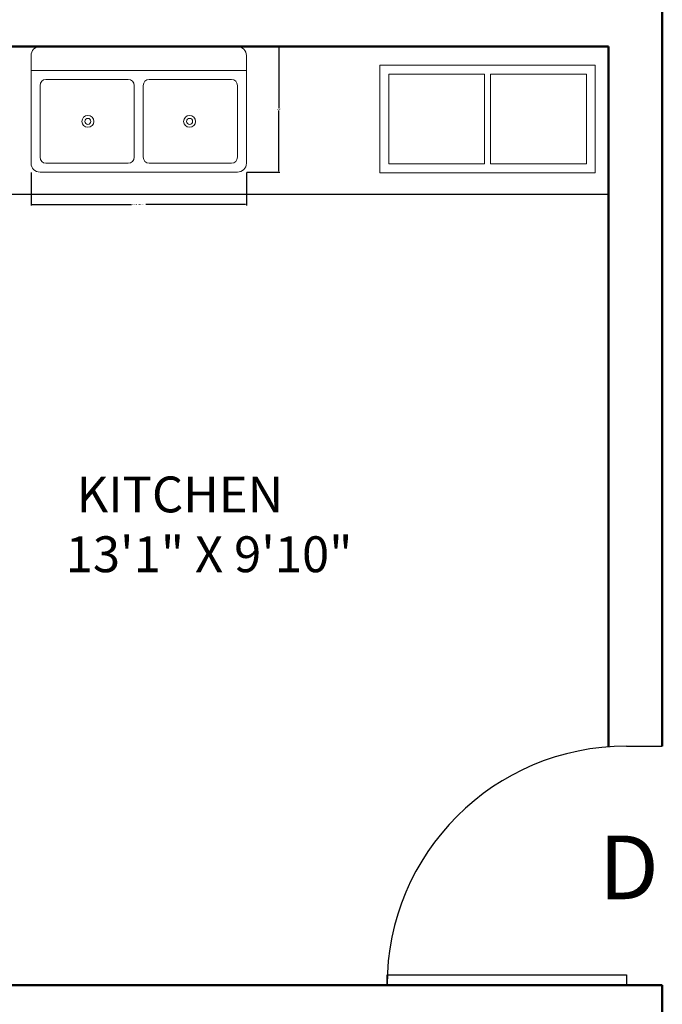
# Model space of a CAD drawing. Units: inches. Extents: x -105 to 1196, y -792 to 119.
# Tile 6 of 23: x 22 to 130, y -285 to -121. Entities that reach past the tile are written whole.
import ezdxf

# ---------------------------------------------------------------- set-up
doc = ezdxf.new("R2010")
doc.units = ezdxf.units.IN
doc.header["$MEASUREMENT"] = 0
for name, color, linetype, lineweight in [('A-ANNO-DIMS', 2, 'Continuous', 18), ('A-ANNO-TEXT', 7, 'Continuous', 25), ('A-AREA-IDEN', 7, 'Continuous', 25), ('A-DOOR', 4, 'Continuous', 25), ('A-FLOR-FIXT', 8, 'Continuous', 18), ('A-GLAZ', 4, 'Continuous', 25), ('A-WALL', 3, 'Continuous', 50)]:
    doc.layers.add(name, color=color, linetype=linetype, lineweight=lineweight)
doc.styles.get("Standard").update_dxf_attribs({"font": 'arial.ttf'})
doc.dimstyles.get("Standard").update_dxf_attribs({"dimtxt": 0.18, "dimasz": 0.18, "dimexe": 0.18, "dimexo": 0.0625, "dimgap": 0.09, "dimtad": 0, "dimtih": 1, "dimtoh": 1, "dimdec": 1, "dimzin": 0, "dimdsep": 46, "dimlunit": 4, "dimtxsty": 'Standard', "dimcen": 0.09, "dimadec": 0, "dimazin": 0, "dimtfac": 1, "dimtdec": 1, "dimtofl": 0, "dimtmove": 0, "dimatfit": 3, "dimfxl": 1, "dimtolj": 1, "dimtzin": 0, "dimarcsym": 0})

# ---------------------------------------------------------------- blocks, each defined once
blk = doc.blocks.new('*U4')
for p, q in [((0, 0), (0, -6)), ((40, 0), (40, -6))]:
    blk.add_line(p, q)
blk.add_lwpolyline([(0, 0), (0, 40), (1.75, 40), (1.75, 0)], close=True)
blk.add_arc((0, 0), 40, 0, 90)
blk = doc.blocks.new('Sink-double - 36 in top')
for p, q in [((-18, -4), (18, -4)), ((-0.75, -18.5), (-0.75, -6.5)), ((0.75, -6.5), (0.75, -18.5))]:
    blk.add_line(p, q)
for points in [[(-16.5, 0), (16.5, 0)], [(-18, -19.5), (-18, -1.5)], [(18, -1.5), (18, -19.5)], [(-16.5, -18.5), (-16.5, -6.5)], [(-15.5, -5.5), (-1.75, -5.5)], [(1.75, -5.5), (15.5, -5.5)], [(16.5, -6.5), (16.5, -18.5)], [(-1.75, -19.5), (-15.5, -19.5)], [(15.5, -19.5), (1.75, -19.5)], [(16.5, -21), (-16.5, -21)]]:
    blk.add_lwpolyline(points)
for centre, radius in [((-8.5, -12.5), 1), ((8.5, -12.5), 1), ((-8.5, -12.5), 0.5), ((8.5, -12.5), 0.5)]:
    blk.add_circle(centre, radius)
for centre, radius, start, end in [((-16.5, -1.5), 1.5, 90, 180), ((16.5, -1.5), 1.5, 0, 90), ((-15.5, -6.5), 1, 90, 180), ((-1.75, -6.5), 1, 0, 90), ((1.75, -6.5), 1, 90, 180), ((15.5, -6.5), 1, 0, 90), ((-16.5, -19.5), 1.5, 180, 270), ((-15.5, -18.5), 1, 180, 270), ((-1.75, -18.5), 1, 270, 0), ((1.75, -18.5), 1, 180, 270), ((15.5, -18.5), 1, 270, 0), ((16.5, -19.5), 1.5, 270, 0)]:
    blk.add_arc(centre, radius, start, end)
blk = doc.blocks.new('Wall Cabinet - 18 x 36 in front')
for p, q in [((17.5, -1.5), (17.5, -16.5)), ((18.5, -16.5), (18.5, -1.5))]:
    blk.add_line(p, q)
blk.add_lwpolyline([(0, -18), (0, 0), (36, 0), (36, -18)], close=True)
for points in [[(17.5, -16.5), (1.5, -16.5), (1.5, -1.5), (17.5, -1.5)], [(18.5, -1.5), (34.5, -1.5), (34.5, -16.5), (18.5, -16.5)]]:
    blk.add_lwpolyline(points)
blk = doc.blocks.new('*D87')
at = {"layer": 'A-ANNO-DIMS', "color": 0, "lineweight": -2, "transparency": 16777216}
for p, q in [((24.24, -146.29), (24.24, -151.81)), ((60.24, -146.29), (60.24, -151.81)), ((24.42, -151.63), (41.04, -151.63)), ((60.06, -151.63), (43.45, -151.63))]:
    blk.add_line(p, q, dxfattribs=at)
at = {"layer": 'A-ANNO-DIMS', "color": 0, "transparency": 16777216}
for points in [[(24.42, -151.6), (24.42, -151.66), (24.24, -151.63)], [(60.06, -151.6), (60.06, -151.66), (60.24, -151.63)]]:
    blk.add_solid(points, dxfattribs=at)
at = {"layer": 'Defpoints', "color": 0, "transparency": 16777216}
for p in [(24.24, -146.23), (60.24, -146.23), (60.24, -151.63)]:
    blk.add_point(p, dxfattribs=at)
at = {"layer": 'A-ANNO-DIMS', "color": 0, "transparency": 16777216, "insert": (42.24, -151.63), "char_height": 0.18, "attachment_point": 5}
blk.add_mtext('\\A1;DOUBLE SINK 3\'-0"', dxfattribs=at)
blk = doc.blocks.new('*D88')
at = {"layer": 'A-ANNO-DIMS', "color": 0, "lineweight": -2, "transparency": 16777216}
for p, q in [((60.31, -125.23), (65.82, -125.23)), ((65.64, -125.41), (65.64, -135.55)), ((65.64, -146.05), (65.64, -135.91)), ((60.31, -146.23), (65.82, -146.23))]:
    blk.add_line(p, q, dxfattribs=at)
at = {"layer": 'A-ANNO-DIMS', "color": 0, "transparency": 16777216}
for points in [[(65.61, -125.41), (65.67, -125.41), (65.64, -125.23)], [(65.61, -146.05), (65.67, -146.05), (65.64, -146.23)]]:
    blk.add_solid(points, dxfattribs=at)
at = {"layer": 'Defpoints', "color": 0, "transparency": 16777216}
for p in [(60.24, -125.23), (65.64, -125.23), (60.24, -146.23)]:
    blk.add_point(p, dxfattribs=at)
at = {"layer": 'A-ANNO-DIMS', "color": 0, "transparency": 16777216, "insert": (65.64, -135.73), "char_height": 0.18, "attachment_point": 5}
blk.add_mtext('\\A1;1\'-9"', dxfattribs=at)

msp = doc.modelspace()

# ---------------------------------------------------------------- linework, layer by layer
at = {"layer": 'A-GLAZ'}
msp.add_line((120.74, -149.97), (-5.49, -149.97), dxfattribs=at)
at = {"layer": 'A-WALL'}
for p, q in [((129.74, -116.23), (129.74, -242.23)), ((-36.26, -125.23), (120.74, -125.23)), ((120.74, -125.23), (120.74, -242.34)), ((129.74, -219.23), (129.74, -228.23)), ((-36.26, -282.23), (129.74, -282.23)), ((129.74, -282.23), (129.74, -291.23))]:
    msp.add_line(p, q, dxfattribs=at)

# ---------------------------------------------------------------- block references
at = {"layer": 'A-DOOR', "rotation": 90}
msp.add_blockref('*U4', (123.74, -282.23), dxfattribs=at)
at = {"layer": 'A-FLOR-FIXT'}
for name, p in [('Sink-double - 36 in top', (42.24, -125.23)), ('Wall Cabinet - 18 x 36 in front', (82.55, -128.32))]:
    msp.add_blockref(name, p, dxfattribs=at)

# ---------------------------------------------------------------- texts
at = {"layer": 'A-ANNO-TEXT'}
msp.add_text('D', height=10.64, dxfattribs=at).set_placement((119.17, -267.83))
at = {"layer": 'A-AREA-IDEN', "insert": (30.03, -197.13), "char_height": 6, "attachment_point": 1}
msp.add_mtext_dynamic_manual_height_columns(' KITCHEN\\P13\'1" X 9\'10"', width=59.5623, gutter_width=1, heights=[0], dxfattribs=at)

# ---------------------------------------------------------------- dimensions: what is measured, and where the dimension line sits
at = {"layer": 'A-ANNO-DIMS'}
dim = msp.add_linear_dim(base=(65.64, -125.23), p1=(60.24, -146.23), p2=(60.24, -125.23), angle=90, dimstyle='Standard', override={"dimdec": 1, "dimlfac": 1, "dimrnd": 0, "dimzin": 1, "dimdsep": 46, "dimlunit": 4, "dimfrac": 2}, dxfattribs=at)
dim.commit()
dim.dimension.update_dxf_attribs({"geometry": '*D88', "text_midpoint": (65.64, -135.73)})
dim = msp.add_linear_dim(base=(60.24, -151.63), p1=(24.24, -146.23), p2=(60.24, -146.23), text='DOUBLE SINK <>', dimstyle='Standard', override={"dimdec": 1, "dimlfac": 1, "dimrnd": 0, "dimzin": 1, "dimdsep": 46, "dimlunit": 4, "dimfrac": 2}, dxfattribs=at)
dim.commit()
dim.dimension.update_dxf_attribs({"geometry": '*D87', "text_midpoint": (42.24, -151.63)})

doc.saveas('drawing.dxf')
